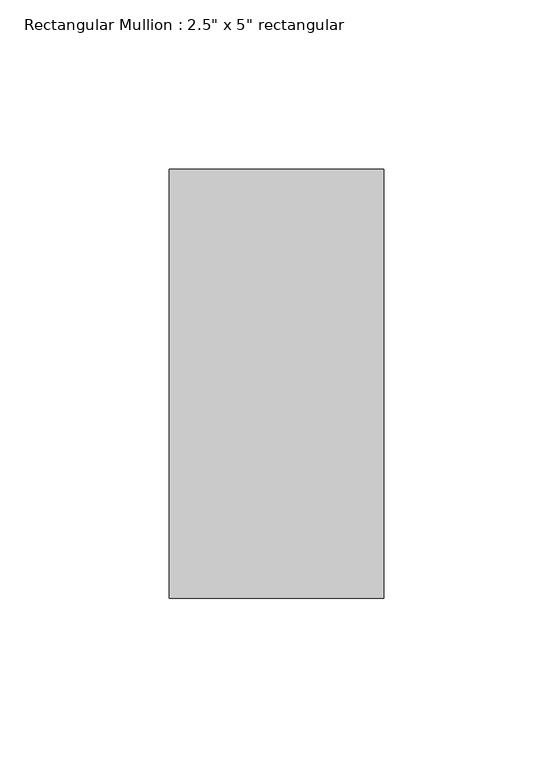
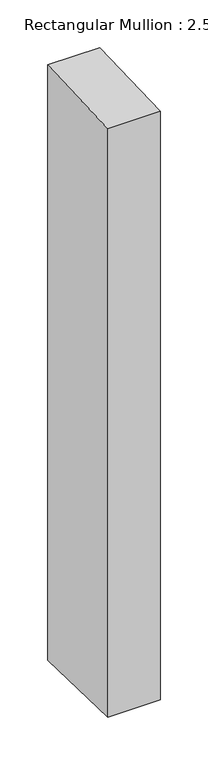
"""IFC4 building model written with IfcOpenShell, lengths in millimetres: member geometry."""

from ifc_helpers import new_model, si_unit, frame, origin, place, context, project, spatial, polyline, outline, extrude, source, transform, mapped, element, save


def member_0d2ca346(model_context):
    return source(origin(), model_context, "Body", "SweptSolid", [
        extrude(outline(polyline([(-63.5, -2.3994633), (63.5, 2.3994633), (63.5, -762.2019944), (-63.5, -758.0444448), (-63.5, -2.3994633)])), frame((-63.5, 0.0, 0.0), z_axis=(1.0, 0.0, 0.0), x_axis=(0.0, 1.0, 0.0)), (0.0, 0.0, 1.0), 63.5),
    ])


if __name__ == "__main__":
    model = new_model("IFC4")
    model_context = context("Model", 3, world=origin())
    ifc_project = project(units=[si_unit("LENGTHUNIT", "METRE", prefix="MILLI")], contexts=[model_context])
    site = spatial("IfcSite", under=ifc_project)
    building = spatial("IfcBuilding", under=site)
    placement = place(None, origin())
    member_shape = member_0d2ca346(model_context)
    element("IfcMember", 1, ObjectType="Rectangular Mullion : 2.5\" x 5\" rectangular", at=placement, inside=building, context=model_context, shape_type="MappedRepresentation", body=[
        mapped(member_shape, transform((0.0, 0.0, 0.0), x_axis=(1.0, 0.0, 0.0), y_axis=(0.0, 1.0, 0.0), z_axis=(0.0, 0.0, 1.0))),
    ])
    save(model, "model.ifc")

# Revit data of these elements
# Type "Rectangular Mullion : 2.5\" x 5\" rectangular"
#   built-in parameter 1007304 = 0.416667 (stored number, unit not read)
#   built-in parameter 1007301 = 0.104167 (stored number, unit not read)
#   built-in parameter 1007300 = 0.104167 (stored number, unit not read)
# Element 1 (IfcMember, "Rectangular Mullion : 2.5\" x 5\" rectangular")
#   Materials on its faces: "Aluminum"
# Materials
#   "Aluminum": class "Metal", colour RGB 247 247 247, transparency 0, Description = "Aluminum 6061", Cost = 0
